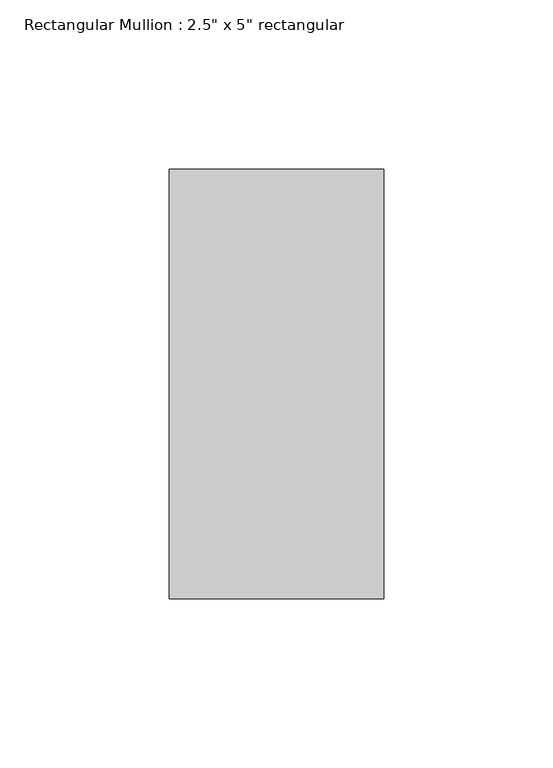
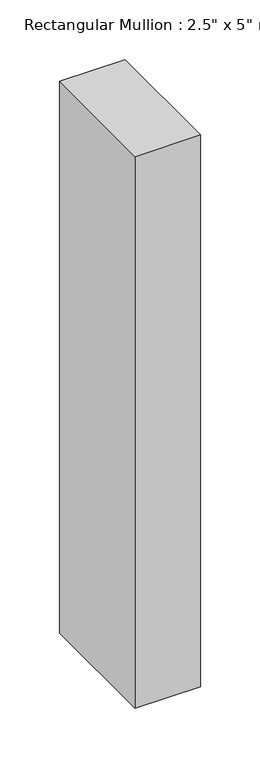
"""IFC4 building model written with IfcOpenShell, lengths in millimetres: member geometry."""

from ifc_helpers import new_model, si_unit, frame, origin, place, context, project, spatial, polyline, outline, extrude, source, transform, mapped, element, save


def member_6103f85b(model_context):
    return source(origin(), model_context, "Body", "SweptSolid", [
        extrude(outline(polyline([(31.75, 63.5), (31.75, -63.5), (-31.75, -63.5), (-31.75, 63.5), (31.75, 63.5)])), frame((0.0, 0.0, -565.15), z_axis=(0.0, 0.0, 1.0), x_axis=(1.0, 0.0, 0.0)), (0.0, 0.0, 1.0), 565.15),
    ])


if __name__ == "__main__":
    model = new_model("IFC4")
    model_context = context("Model", 3, world=origin())
    ifc_project = project(units=[si_unit("LENGTHUNIT", "METRE", prefix="MILLI")], contexts=[model_context])
    site = spatial("IfcSite", under=ifc_project)
    building = spatial("IfcBuilding", under=site)
    placement = place(None, origin())
    member_shape = member_6103f85b(model_context)
    element("IfcMember", 1, ObjectType="Rectangular Mullion : 2.5\" x 5\" rectangular", at=placement, inside=building, context=model_context, shape_type="MappedRepresentation", body=[
        mapped(member_shape, transform((0.0, 0.0, 0.0), x_axis=(1.0, 0.0, 0.0), y_axis=(0.0, 1.0, 0.0), z_axis=(0.0, 0.0, 1.0))),
    ])
    save(model, "model.ifc")

# Revit data of these elements
# Type "Rectangular Mullion : 2.5\" x 5\" rectangular"
#   built-in parameter 1007304 = 0.416667 (stored number, unit not read)
#   built-in parameter 1007301 = 0.104167 (stored number, unit not read)
#   built-in parameter 1007300 = 0.104167 (stored number, unit not read)
# Element 1 (IfcMember, "Rectangular Mullion : 2.5\" x 5\" rectangular")
#   Materials on its faces: "Aluminum"
# Materials
#   "Aluminum": class "Metal", colour RGB 247 247 247, transparency 0, Description = "Aluminum 6061", Cost = 0
